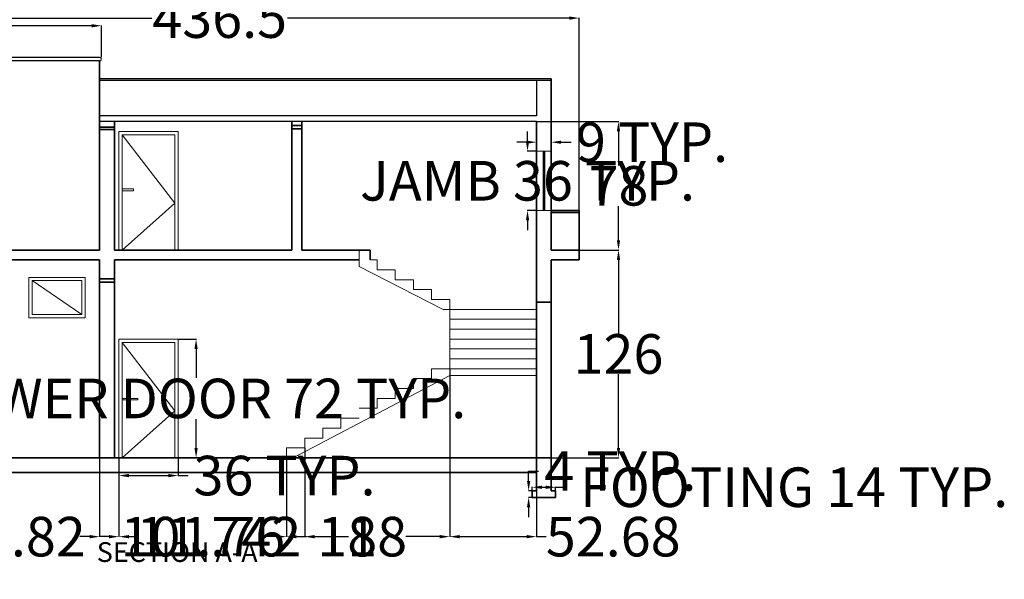
# Model space of a CAD drawing. Units: inches. Extents: x -15 to 1815, y 1023 to 2303.
# Tile 7 of 8: x 1217 to 1815, y 1433 to 1773. Entities that reach past the tile are written whole.
import ezdxf

# ---------------------------------------------------------------- set-up
doc = ezdxf.new("R2010")
doc.units = ezdxf.units.IN
doc.header["$MEASUREMENT"] = 0
for name, color, linetype, lineweight in [('A-ANNO-DIMS', 2, 'Continuous', 18), ('A-ANNO-TEXT', 7, 'Continuous', 25), ('A-DOOR', 3, 'Continuous', 18), ('A-FLOR', 7, 'Continuous', 35), ('A-FLOR-STRS', 3, 'Continuous', 18), ('A-GLAZ', 4, 'Continuous', 18), ('A-ROOF', 7, 'Continuous', 25), ('A-SECT', 7, 'Continuous', 35), ('S-FNDN', 7, 'Continuous', 35)]:
    doc.layers.add(name, color=color, linetype=linetype, lineweight=lineweight)
doc.styles.get("Standard").update_dxf_attribs({"font": 'arial.ttf'})
doc.dimstyles.get("Standard").update_dxf_attribs({"dimtxt": 24, "dimasz": 6, "dimexe": 0.18, "dimexo": 0.0625, "dimgap": 0.09, "dimtad": 0, "dimtih": 1, "dimtoh": 1, "dimdec": 0, "dimzin": 0, "dimdsep": 46, "dimlunit": 3, "dimtxsty": 'Standard', "dimcen": 0.09, "dimadec": 0, "dimazin": 0, "dimtfac": 1, "dimtdec": 0, "dimtofl": 0, "dimtmove": 0, "dimatfit": 3, "dimfxl": 1, "dimtolj": 1, "dimtzin": 0, "dimarcsym": 0})

# ---------------------------------------------------------------- blocks, each defined once
blk = doc.blocks.new('DOOR-36-SEC-LEVER')
for p, q in [((2, 70), (34, 28.45)), ((34, 28.45), (2, 0)), ((2, 2), (2, 0)), ((34, 2), (34, 0))]:
    blk.add_line(p, q)
for points in [[(0, 0), (36, 0), (36, 72), (0, 72)], [(2, 36), (11.36, 36), (11.36, 35.17), (2, 35.17)]]:
    blk.add_lwpolyline(points, close=True)
blk.add_lwpolyline([(34, 2), (34, 70), (2, 70), (2, 2)])
blk = doc.blocks.new('DOOR-36-SEC-RETURN-LEVER')
for p, q in [((2, 70), (34, 28.45)), ((8.91, 37.23), (2, 37.23)), ((8.91, 36), (2, 36)), ((8.91, 36), (8.91, 37.23)), ((34, 28.45), (2, 0)), ((2, 2), (2, 0)), ((34, 2), (34, 0))]:
    blk.add_line(p, q)
for points in [[(0, 0), (36, 0), (36, 72), (0, 72)], [(2, 36), (8.91, 36), (8.91, 36), (2, 36)]]:
    blk.add_lwpolyline(points, close=True)
blk.add_lwpolyline([(34, 2), (34, 70), (2, 70), (2, 2)])
blk = doc.blocks.new('WIN-AWNING-ELEV')
blk.add_line((32.26, 2), (2, 22.53))
for points in [[(0, 24.53), (34.26, 24.53), (34.26, 0), (0, 0)], [(2, 22.53), (32.26, 22.53), (32.26, 2), (2, 2)]]:
    blk.add_lwpolyline(points, close=True)
blk = doc.blocks.new('WIN-36-JAMB-SEC')
for p, q in [((4, 36.04), (4, 0)), ((4.5, 36.04), (4.5, 0)), ((5, 36.04), (5, 0))]:
    blk.add_line(p, q)
blk.add_lwpolyline([(9, 0), (0, 0), (0, 36.04), (9, 36.04)], close=True)
blk = doc.blocks.new('COPING-ROUND-END')
for p, q in [((1.07, 2.13), (126.89, 2.13)), ((1.07, 0), (126.89, 0))]:
    blk.add_line(p, q)
for centre, start, end in [((1.07, 1.07), 90, 270), ((126.89, 1.07), 270, 90)]:
    blk.add_arc(centre, 1.07, start, end)
blk = doc.blocks.new('FOOTING-STRIP-SECTION')
for p, q in [((0, 0), (0, 3.98)), ((0, 3.98), (2.61, 3.98)), ((14.22, 0), (0, 0)), ((14.22, 3.98), (11.61, 3.98)), ((14.22, 0), (14.22, 3.98))]:
    blk.add_line(p, q)
blk = doc.blocks.new('*D45')
at = {"layer": 'A-ANNO-DIMS', "color": 0, "lineweight": -2, "transparency": 16777216}
for p, q in [((1138.43, 1750.02), (1138.43, 1769.34)), ((1266.44, 1750.02), (1266.44, 1769.34)), ((1138.43, 1769.16), (1132.43, 1769.16)), ((1260.44, 1769.16), (1144.43, 1769.16))]:
    blk.add_line(p, q, dxfattribs=at)
at = {"layer": 'A-ANNO-DIMS', "color": 0, "transparency": 16777216}
for points in [[(1144.43, 1770.16), (1144.43, 1768.16), (1138.43, 1769.16)], [(1260.44, 1770.16), (1260.44, 1768.16), (1266.44, 1769.16)]]:
    blk.add_solid(points, dxfattribs=at)
at = {"layer": 'Defpoints', "color": 0, "transparency": 16777216}
for p in [(1138.43, 1769.16), (1138.43, 1749.96), (1266.44, 1749.96)]:
    blk.add_point(p, dxfattribs=at)
at = {"layer": 'A-ANNO-DIMS', "color": 0, "transparency": 16777216, "insert": (993.96, 1769.16), "char_height": 24, "attachment_point": 5}
blk.add_mtext('\\A1;COPING 128 TYP.', dxfattribs=at)
blk = doc.blocks.new('*D47')
at = {"layer": 'A-ANNO-DIMS', "color": 0, "lineweight": -2, "transparency": 16777216}
for p, q in [((1527.89, 1487.12), (1527.89, 1489.37)), ((1533.89, 1489.19), (1536.11, 1489.19)), ((1542.11, 1487.12), (1542.11, 1489.37)), ((1542.11, 1489.19), (1548.11, 1489.19))]:
    blk.add_line(p, q, dxfattribs=at)
at = {"layer": 'A-ANNO-DIMS', "color": 0, "transparency": 16777216}
for points in [[(1533.89, 1490.19), (1533.89, 1488.19), (1527.89, 1489.19)], [(1536.11, 1490.19), (1536.11, 1488.19), (1542.11, 1489.19)]]:
    blk.add_solid(points, dxfattribs=at)
at = {"layer": 'Defpoints', "color": 0, "transparency": 16777216}
for p in [(1542.11, 1489.19), (1527.89, 1487.06), (1542.11, 1487.06)]:
    blk.add_point(p, dxfattribs=at)
at = {"layer": 'A-ANNO-DIMS', "color": 0, "transparency": 16777216, "insert": (1686.95, 1489.19), "char_height": 24, "attachment_point": 5}
blk.add_mtext('\\A1;FOOTING 14 TYP.', dxfattribs=at)
blk = doc.blocks.new('*D48')
at = {"layer": 'A-ANNO-DIMS', "color": 0, "lineweight": -2, "transparency": 16777216}
for p, q in [((1525.76, 1493.06), (1525.76, 1499.06)), ((1525.76, 1499.06), (1531.76, 1499.06)), ((1527.83, 1487.06), (1525.58, 1487.06)), ((1527.83, 1483.08), (1525.58, 1483.08)), ((1525.76, 1477.08), (1525.76, 1471.08))]:
    blk.add_line(p, q, dxfattribs=at)
at = {"layer": 'A-ANNO-DIMS', "color": 0, "transparency": 16777216}
for points in [[(1524.76, 1493.06), (1526.76, 1493.06), (1525.76, 1487.06)], [(1524.76, 1477.08), (1526.76, 1477.08), (1525.76, 1483.08)]]:
    blk.add_solid(points, dxfattribs=at)
at = {"layer": 'Defpoints', "color": 0, "transparency": 16777216}
for p in [(1525.76, 1487.06), (1527.89, 1487.06), (1527.89, 1483.08)]:
    blk.add_point(p, dxfattribs=at)
at = {"layer": 'A-ANNO-DIMS', "color": 0, "transparency": 16777216, "insert": (1581.42, 1499.06), "char_height": 24, "attachment_point": 5}
blk.add_mtext('\\A1;4 TYP.', dxfattribs=at)
blk = doc.blocks.new('*D49')
at = {"layer": 'A-ANNO-DIMS', "color": 0, "lineweight": -2, "transparency": 16777216}
for p, q in [((1313.13, 1579.08), (1324.05, 1579.08)), ((1323.87, 1573.08), (1323.87, 1555.58)), ((1323.87, 1513.08), (1323.87, 1530.57)), ((1313.13, 1507.08), (1324.05, 1507.08))]:
    blk.add_line(p, q, dxfattribs=at)
at = {"layer": 'A-ANNO-DIMS', "color": 0, "transparency": 16777216}
for points in [[(1322.87, 1573.08), (1324.87, 1573.08), (1323.87, 1579.08)], [(1322.87, 1513.08), (1324.87, 1513.08), (1323.87, 1507.08)]]:
    blk.add_solid(points, dxfattribs=at)
at = {"layer": 'Defpoints', "color": 0, "transparency": 16777216}
for p in [(1313.07, 1579.08), (1323.87, 1579.08), (1313.07, 1507.08)]:
    blk.add_point(p, dxfattribs=at)
at = {"layer": 'A-ANNO-DIMS', "color": 0, "transparency": 16777216, "insert": (1323.87, 1543.08), "char_height": 24, "attachment_point": 5}
blk.add_mtext('\\A1;LOWER DOOR 72 TYP.', dxfattribs=at)
blk = doc.blocks.new('*D50')
at = {"layer": 'A-ANNO-DIMS', "color": 0, "lineweight": -2, "transparency": 16777216}
for p, q in [((1277.07, 1507.01), (1277.07, 1496.1)), ((1313.07, 1507.01), (1313.07, 1496.1)), ((1283.07, 1496.28), (1307.07, 1496.28)), ((1313.07, 1496.28), (1319.07, 1496.28))]:
    blk.add_line(p, q, dxfattribs=at)
at = {"layer": 'A-ANNO-DIMS', "color": 0, "transparency": 16777216}
for points in [[(1283.07, 1497.28), (1283.07, 1495.28), (1277.07, 1496.28)], [(1307.07, 1497.28), (1307.07, 1495.28), (1313.07, 1496.28)]]:
    blk.add_solid(points, dxfattribs=at)
at = {"layer": 'Defpoints', "color": 0, "transparency": 16777216}
for p in [(1277.07, 1507.08), (1313.07, 1507.08), (1313.07, 1496.28)]:
    blk.add_point(p, dxfattribs=at)
at = {"layer": 'A-ANNO-DIMS', "color": 0, "transparency": 16777216, "insert": (1377.56, 1496.28), "char_height": 24, "attachment_point": 5}
blk.add_mtext('\\A1;36 TYP.', dxfattribs=at)
blk = doc.blocks.new('*D55')
at = {"layer": 'A-ANNO-DIMS', "color": 0, "lineweight": -2, "transparency": 16777216}
for p, q in [((1525.09, 1699.11), (1525.09, 1705.11)), ((1530.44, 1693.11), (1524.91, 1693.11)), ((1530.44, 1657.08), (1524.91, 1657.08)), ((1525.09, 1651.08), (1525.09, 1645.08))]:
    blk.add_line(p, q, dxfattribs=at)
at = {"layer": 'A-ANNO-DIMS', "color": 0, "transparency": 16777216}
for points in [[(1524.09, 1699.11), (1526.09, 1699.11), (1525.09, 1693.11)], [(1524.09, 1651.08), (1526.09, 1651.08), (1525.09, 1657.08)]]:
    blk.add_solid(points, dxfattribs=at)
at = {"layer": 'Defpoints', "color": 0, "transparency": 16777216}
for p in [(1525.09, 1693.11), (1530.5, 1693.11), (1530.5, 1657.08)]:
    blk.add_point(p, dxfattribs=at)
at = {"layer": 'A-ANNO-DIMS', "color": 0, "transparency": 16777216, "insert": (1525.09, 1675.1), "char_height": 24, "attachment_point": 5}
blk.add_mtext('\\A1;JAMB 36 TYP.', dxfattribs=at)
blk = doc.blocks.new('*D56')
at = {"layer": 'A-ANNO-DIMS', "color": 0, "lineweight": -2, "transparency": 16777216}
for p, q in [((1524.5, 1698.52), (1518.5, 1698.52)), ((1530.5, 1693.18), (1530.5, 1698.7)), ((1539.5, 1693.18), (1539.5, 1698.7)), ((1545.5, 1698.52), (1551.5, 1698.52))]:
    blk.add_line(p, q, dxfattribs=at)
at = {"layer": 'A-ANNO-DIMS', "color": 0, "transparency": 16777216}
for points in [[(1524.5, 1699.52), (1524.5, 1697.52), (1530.5, 1698.52)], [(1545.5, 1699.52), (1545.5, 1697.52), (1539.5, 1698.52)]]:
    blk.add_solid(points, dxfattribs=at)
at = {"layer": 'Defpoints', "color": 0, "transparency": 16777216}
for p in [(1539.5, 1698.52), (1530.5, 1693.11), (1539.5, 1693.11)]:
    blk.add_point(p, dxfattribs=at)
at = {"layer": 'A-ANNO-DIMS', "color": 0, "transparency": 16777216, "insert": (1600.68, 1698.52), "char_height": 24, "attachment_point": 5}
blk.add_mtext('\\A1;9 TYP.', dxfattribs=at)
blk = doc.blocks.new('*D103')
at = {"layer": 'A-ANNO-DIMS', "color": 0, "lineweight": -2, "transparency": 16777216}
for p, q in [((1119.96, 1657.14), (1119.96, 1773.99)), ((1125.96, 1773.81), (1297.05, 1773.81)), ((1550.46, 1773.81), (1379.37, 1773.81)), ((1556.46, 1657.14), (1556.46, 1773.99))]:
    blk.add_line(p, q, dxfattribs=at)
at = {"layer": 'A-ANNO-DIMS', "color": 0, "transparency": 16777216}
for points in [[(1125.96, 1774.81), (1125.96, 1772.81), (1119.96, 1773.81)], [(1550.46, 1774.81), (1550.46, 1772.81), (1556.46, 1773.81)]]:
    blk.add_solid(points, dxfattribs=at)
at = {"layer": 'Defpoints', "color": 0, "transparency": 16777216}
for p in [(1556.46, 1773.81), (1119.96, 1657.08), (1556.46, 1657.08)]:
    blk.add_point(p, dxfattribs=at)
at = {"layer": 'A-ANNO-DIMS', "color": 0, "transparency": 16777216, "insert": (1338.21, 1773.81), "char_height": 24, "attachment_point": 5}
blk.add_mtext('\\A1;436.5', dxfattribs=at)
blk = doc.blocks.new('*D105')
at = {"layer": 'A-ANNO-DIMS', "color": 0, "lineweight": -2, "transparency": 16777216}
for p, q in [((1556.52, 1633.08), (1580.49, 1633.08)), ((1580.31, 1627.08), (1580.31, 1582.42)), ((1580.31, 1513.08), (1580.31, 1557.73)), ((1539.56, 1507.08), (1580.49, 1507.08))]:
    blk.add_line(p, q, dxfattribs=at)
at = {"layer": 'A-ANNO-DIMS', "color": 0, "transparency": 16777216}
for points in [[(1579.31, 1627.08), (1581.31, 1627.08), (1580.31, 1633.08)], [(1579.31, 1513.08), (1581.31, 1513.08), (1580.31, 1507.08)]]:
    blk.add_solid(points, dxfattribs=at)
at = {"layer": 'Defpoints', "color": 0, "transparency": 16777216}
for p in [(1556.46, 1633.08), (1580.31, 1633.08), (1539.5, 1507.08)]:
    blk.add_point(p, dxfattribs=at)
at = {"layer": 'A-ANNO-DIMS', "color": 0, "transparency": 16777216, "insert": (1580.31, 1570.08), "char_height": 24, "attachment_point": 5}
blk.add_mtext('\\A1;126', dxfattribs=at)
blk = doc.blocks.new('*D106')
at = {"layer": 'A-ANNO-DIMS', "color": 0, "lineweight": -2, "transparency": 16777216}
for p, q in [((1530.56, 1711.08), (1580.49, 1711.08)), ((1580.31, 1705.08), (1580.31, 1684.42)), ((1580.31, 1639.08), (1580.31, 1659.73)), ((1539.56, 1633.08), (1580.49, 1633.08))]:
    blk.add_line(p, q, dxfattribs=at)
at = {"layer": 'A-ANNO-DIMS', "color": 0, "transparency": 16777216}
for points in [[(1579.31, 1705.08), (1581.31, 1705.08), (1580.31, 1711.08)], [(1579.31, 1639.08), (1581.31, 1639.08), (1580.31, 1633.08)]]:
    blk.add_solid(points, dxfattribs=at)
at = {"layer": 'Defpoints', "color": 0, "transparency": 16777216}
for p in [(1530.5, 1711.08), (1580.31, 1711.08), (1539.5, 1633.08)]:
    blk.add_point(p, dxfattribs=at)
at = {"layer": 'A-ANNO-DIMS', "color": 0, "transparency": 16777216, "insert": (1580.31, 1672.08), "char_height": 24, "attachment_point": 5}
blk.add_mtext('\\A1;78', dxfattribs=at)
blk = doc.blocks.new('*D107')
at = {"layer": 'A-ANNO-DIMS', "color": 0, "lineweight": -2, "transparency": 16777216}
for p, q in [((1148.5, 1507.01), (1148.5, 1459.05)), ((1265.32, 1507.01), (1265.32, 1459.05)), ((1154.5, 1459.23), (1158.26, 1459.23)), ((1259.32, 1459.23), (1255.57, 1459.23))]:
    blk.add_line(p, q, dxfattribs=at)
at = {"layer": 'A-ANNO-DIMS', "color": 0, "transparency": 16777216}
for points in [[(1154.5, 1460.23), (1154.5, 1458.23), (1148.5, 1459.23)], [(1259.32, 1460.23), (1259.32, 1458.23), (1265.32, 1459.23)]]:
    blk.add_solid(points, dxfattribs=at)
at = {"layer": 'Defpoints', "color": 0, "transparency": 16777216}
for p in [(1148.5, 1507.08), (1265.32, 1507.08), (1265.32, 1459.23)]:
    blk.add_point(p, dxfattribs=at)
at = {"layer": 'A-ANNO-DIMS', "color": 0, "transparency": 16777216, "insert": (1206.91, 1459.23), "char_height": 24, "attachment_point": 5}
blk.add_mtext('\\A1;116.82', dxfattribs=at)
blk = doc.blocks.new('*D108')
at = {"layer": 'A-ANNO-DIMS', "color": 0, "lineweight": -2, "transparency": 16777216}
for p, q in [((1265.32, 1507.01), (1265.32, 1459.05)), ((1277.07, 1507.01), (1277.07, 1459.05)), ((1259.32, 1459.23), (1253.32, 1459.23)), ((1283.07, 1459.23), (1289.07, 1459.23))]:
    blk.add_line(p, q, dxfattribs=at)
at = {"layer": 'A-ANNO-DIMS', "color": 0, "transparency": 16777216}
for points in [[(1259.32, 1460.23), (1259.32, 1458.23), (1265.32, 1459.23)], [(1283.07, 1460.23), (1283.07, 1458.23), (1277.07, 1459.23)]]:
    blk.add_solid(points, dxfattribs=at)
at = {"layer": 'Defpoints', "color": 0, "transparency": 16777216}
for p in [(1265.32, 1507.08), (1277.07, 1507.08), (1277.07, 1459.23)]:
    blk.add_point(p, dxfattribs=at)
at = {"layer": 'A-ANNO-DIMS', "color": 0, "transparency": 16777216, "insert": (1337.72, 1459.23), "char_height": 24, "attachment_point": 5}
blk.add_mtext('\\A1;11.742', dxfattribs=at)
blk = doc.blocks.new('*D109')
at = {"layer": 'A-ANNO-DIMS', "color": 0, "lineweight": -2, "transparency": 16777216}
for p, q in [((1277.065913, 1507.014849), (1277.065913, 1459.047349)), ((1378.822077, 1507.014849), (1378.822077, 1459.047349)), ((1271.065913, 1459.227349), (1265.065913, 1459.227349)), ((1384.822077, 1459.227349), (1390.822077, 1459.227349))]:
    blk.add_line(p, q, dxfattribs=at)
at = {"layer": 'A-ANNO-DIMS', "color": 0, "transparency": 16777216}
for points in [[(1271.065913, 1460.227349), (1271.065913, 1458.227349), (1277.065913, 1459.227349)], [(1384.822077, 1460.227349), (1384.822077, 1458.227349), (1378.822077, 1459.227349)]]:
    blk.add_solid(points, dxfattribs=at)
at = {"layer": 'Defpoints', "color": 0, "transparency": 16777216}
for p in [(1277.065913, 1507.077349), (1378.822077, 1507.077349), (1378.822077, 1459.227349)]:
    blk.add_point(p, dxfattribs=at)
at = {"layer": 'A-ANNO-DIMS', "color": 0, "transparency": 16777216, "insert": (1327.943995, 1459.227349), "char_height": 24, "attachment_point": 5}
blk.add_mtext('\\A1;101.76', dxfattribs=at)
blk = doc.blocks.new('*D110')
at = {"layer": 'A-ANNO-DIMS', "color": 0, "lineweight": -2, "transparency": 16777216}
for p, q in [((1389.82, 1513.01), (1389.82, 1459.05)), ((1378.82, 1507.01), (1378.82, 1459.05)), ((1372.82, 1459.23), (1366.82, 1459.23)), ((1395.82, 1459.23), (1401.82, 1459.23))]:
    blk.add_line(p, q, dxfattribs=at)
at = {"layer": 'A-ANNO-DIMS', "color": 0, "transparency": 16777216}
for points in [[(1372.82, 1460.23), (1372.82, 1458.23), (1378.82, 1459.23)], [(1395.82, 1460.23), (1395.82, 1458.23), (1389.82, 1459.23)]]:
    blk.add_solid(points, dxfattribs=at)
at = {"layer": 'Defpoints', "color": 0, "transparency": 16777216}
for p in [(1389.82, 1513.08), (1378.82, 1507.08), (1389.82, 1459.23)]:
    blk.add_point(p, dxfattribs=at)
at = {"layer": 'A-ANNO-DIMS', "color": 0, "transparency": 16777216, "insert": (1415.66, 1459.23), "char_height": 24, "attachment_point": 5}
blk.add_mtext('\\A1;11', dxfattribs=at)
blk = doc.blocks.new('*D111')
at = {"layer": 'A-ANNO-DIMS', "color": 0, "lineweight": -2, "transparency": 16777216}
for p, q in [((1477.82, 1561.01), (1477.82, 1459.05)), ((1389.82, 1513.01), (1389.82, 1459.05)), ((1395.82, 1459.23), (1416.5, 1459.23)), ((1471.82, 1459.23), (1451.14, 1459.23))]:
    blk.add_line(p, q, dxfattribs=at)
at = {"layer": 'A-ANNO-DIMS', "color": 0, "transparency": 16777216}
for points in [[(1395.82, 1460.23), (1395.82, 1458.23), (1389.82, 1459.23)], [(1471.82, 1460.23), (1471.82, 1458.23), (1477.82, 1459.23)]]:
    blk.add_solid(points, dxfattribs=at)
at = {"layer": 'Defpoints', "color": 0, "transparency": 16777216}
for p in [(1477.82, 1561.08), (1389.82, 1513.08), (1477.82, 1459.23)]:
    blk.add_point(p, dxfattribs=at)
at = {"layer": 'A-ANNO-DIMS', "color": 0, "transparency": 16777216, "insert": (1433.82, 1459.23), "char_height": 24, "attachment_point": 5}
blk.add_mtext('\\A1;88', dxfattribs=at)
blk = doc.blocks.new('*D112')
at = {"layer": 'A-ANNO-DIMS', "color": 0, "lineweight": -2, "transparency": 16777216}
for p, q in [((1477.82, 1561.01), (1477.82, 1459.05)), ((1530.5, 1561.01), (1530.5, 1459.05)), ((1483.82, 1459.23), (1524.5, 1459.23)), ((1530.5, 1459.23), (1536.5, 1459.23))]:
    blk.add_line(p, q, dxfattribs=at)
at = {"layer": 'A-ANNO-DIMS', "color": 0, "transparency": 16777216}
for points in [[(1483.82, 1460.23), (1483.82, 1458.23), (1477.82, 1459.23)], [(1524.5, 1460.23), (1524.5, 1458.23), (1530.5, 1459.23)]]:
    blk.add_solid(points, dxfattribs=at)
at = {"layer": 'Defpoints', "color": 0, "transparency": 16777216}
for p in [(1477.82, 1561.08), (1530.5, 1561.08), (1530.5, 1459.23)]:
    blk.add_point(p, dxfattribs=at)
at = {"layer": 'A-ANNO-DIMS', "color": 0, "transparency": 16777216, "insert": (1577.11, 1459.23), "char_height": 24, "attachment_point": 5}
blk.add_mtext('\\A1;52.68', dxfattribs=at)

msp = doc.modelspace()

# ---------------------------------------------------------------- linework, layer by layer
at = {"layer": 'A-FLOR'}
for p, q in [((1556.4613, 1657.0773), (1539.4997, 1657.0773)), ((1556.4613, 1657.0773), (1539.4997, 1657.0773)), ((1556.4613, 1655.9681), (1539.4997, 1655.9681)), ((1556.4613, 1657.0773), (1556.4613, 1627.0773)), ((1265.3241, 1633.0773), (1139.4997, 1633.0773)), ((1382.0448, 1633.0773), (1274.3241, 1633.0773)), ((1428.66, 1633.0773), (1388.0448, 1633.0773)), ((1429.568, 1633.0773), (1388.9528, 1633.0773)), ((1429.568, 1633.0773), (1429.568, 1627.0773)), ((1556.4613, 1633.0773), (1539.4997, 1633.0773)), ((1265.3241, 1627.0773), (1139.4997, 1627.0773)), ((1422.8221, 1627.0773), (1274.3241, 1627.0773)), ((1556.4613, 1627.0773), (1539.4997, 1627.0773)), ((1265.3241, 1507.0773), (1139.4997, 1507.0773)), ((1539.4997, 1507.0773), (1265.3241, 1507.0773)), ((1265.3241, 1498.0773), (1148.4997, 1498.0773)), ((1530.4997, 1498.0773), (1265.3241, 1498.0773))]:
    msp.add_line(p, q, dxfattribs=at)
at = {"layer": 'A-FLOR-STRS'}
for p, q in [((1422.8221, 1623.0773), (1422.8221, 1633.0773)), ((1433.8221, 1627.0773), (1429.568, 1627.0773)), ((1433.8221, 1621.0773), (1433.8221, 1627.0773)), ((1473.8221, 1597.0773), (1422.8221, 1623.0773)), ((1444.8221, 1621.0773), (1433.8221, 1621.0773)), ((1444.8221, 1615.0773), (1444.8221, 1621.0773)), ((1455.8221, 1615.0773), (1444.8221, 1615.0773)), ((1455.8221, 1609.0773), (1455.8221, 1615.0773)), ((1466.8221, 1609.0773), (1455.8221, 1609.0773)), ((1466.8221, 1603.0773), (1466.8221, 1609.0773)), ((1477.8221, 1603.0773), (1466.8221, 1603.0773)), ((1477.8221, 1597.0773), (1477.8221, 1603.0773)), ((1477.8221, 1597.0773), (1473.8221, 1597.0773)), ((1477.8221, 1597.0773), (1530.4997, 1597.0773)), ((1477.8221, 1561.0773), (1477.8221, 1597.0773)), ((1477.8221, 1591.0773), (1530.4997, 1591.0773)), ((1477.8221, 1585.0773), (1530.4997, 1585.0773)), ((1477.8221, 1579.0773), (1530.4997, 1579.0773)), ((1477.8221, 1573.0773), (1530.4997, 1573.0773)), ((1477.8221, 1567.0773), (1530.4997, 1567.0773)), ((1466.8221, 1555.0773), (1466.8221, 1561.0773)), ((1466.8221, 1561.0773), (1477.8221, 1561.0773)), ((1477.8221, 1561.0773), (1530.4997, 1561.0773)), ((1477.8221, 1557.0773), (1382.8221, 1507.0773)), ((1455.8221, 1549.0773), (1455.8221, 1555.0773)), ((1455.8221, 1555.0773), (1466.8221, 1555.0773)), ((1477.8221, 1557.0773), (1530.4997, 1557.0773)), ((1444.8221, 1543.0773), (1444.8221, 1549.0773)), ((1444.8221, 1549.0773), (1455.8221, 1549.0773)), ((1433.8221, 1537.0773), (1433.8221, 1543.0773)), ((1433.8221, 1543.0773), (1444.8221, 1543.0773)), ((1422.8221, 1537.0773), (1433.8221, 1537.0773)), ((1411.8221, 1525.0773), (1411.8221, 1531.0773)), ((1411.8221, 1531.0773), (1422.8221, 1531.0773)), ((1400.8221, 1519.0773), (1400.8221, 1525.0773)), ((1400.8221, 1525.0773), (1411.8221, 1525.0773)), ((1389.8221, 1513.0773), (1389.8221, 1519.0773)), ((1389.8221, 1519.0773), (1400.8221, 1519.0773)), ((1378.8221, 1507.0773), (1378.8221, 1513.0773)), ((1378.8221, 1513.0773), (1389.8221, 1513.0773))]:
    msp.add_line(p, q, dxfattribs=at)
at = {"layer": 'A-ROOF'}
for p, q in [((1539.4997, 1736.9695), (1265.3241, 1736.9695)), ((1539.4997, 1735.8674), (1265.3241, 1735.8674)), ((1530.4997, 1735.8674), (1530.4997, 1714.6079)), ((1530.4997, 1714.6079), (1265.3241, 1714.6079)), ((1530.4997, 1711.0773), (1265.3241, 1711.0773))]:
    msp.add_line(p, q, dxfattribs=at)
at = {"layer": 'A-SECT'}
for p, q in [((1265.3241, 1711.0773), (1265.3241, 1747.8268)), ((1539.4997, 1736.9695), (1539.4997, 1633.0773)), ((1265.3241, 1711.0773), (1265.3241, 1633.0773)), ((1274.3241, 1711.0773), (1274.3241, 1633.0773)), ((1382.0448, 1711.0773), (1382.0448, 1633.0773)), ((1388.0448, 1711.0773), (1388.0448, 1633.0773)), ((1530.4997, 1711.0773), (1530.4997, 1607.8282)), ((1265.3241, 1627.0773), (1265.3241, 1507.0773)), ((1274.3241, 1627.0773), (1274.3241, 1507.0773)), ((1539.4997, 1627.0773), (1539.4997, 1607.8282)), ((1530.4997, 1607.8282), (1530.4997, 1507.0773)), ((1539.4997, 1607.8282), (1539.4997, 1507.0773)), ((1530.4997, 1601.4023), (1539.4997, 1601.4023))]:
    msp.add_line(p, q, dxfattribs=at)
for points in [[(1265.3241, 1707.6644), (1274.3241, 1707.6644), (1274.3241, 1706.2986), (1265.3241, 1706.2986)], [(1382.0448, 1708.6419), (1388.0448, 1708.6419), (1388.0448, 1706.702), (1382.0448, 1706.702)], [(1265.3241, 1615.7133), (1274.3241, 1615.7133), (1274.3241, 1613.5418), (1265.3241, 1613.5418)]]:
    msp.add_lwpolyline(points, close=True, dxfattribs=at)
at = {"layer": 'S-FNDN'}
for p, q in [((1530.4997, 1582.655), (1530.4997, 1487.0609)), ((1530.4997, 1582.655), (1530.4997, 1487.0609)), ((1539.4997, 1582.655), (1539.4997, 1487.0609)), ((1539.4997, 1483.0773), (1527.8895, 1483.0773))]:
    msp.add_line(p, q, dxfattribs=at)

# ---------------------------------------------------------------- block references
at = {"layer": 'A-DOOR'}
for name, p in [('DOOR-36-SEC-RETURN-LEVER', (1277.0659, 1633.0773)), ('DOOR-36-SEC-LEVER', (1277.0659, 1507.0773))]:
    msp.add_blockref(name, p, dxfattribs=at)
at = {"layer": 'A-GLAZ'}
for name, p in [('WIN-36-JAMB-SEC', (1530.4997, 1657.0773)), ('WIN-AWNING-ELEV', (1222.3022, 1592.0097))]:
    msp.add_blockref(name, p, dxfattribs=at)
at = {"layer": 'A-ROOF', "rotation": 180}
msp.add_blockref('COPING-ROUND-END', (1266.39, 1749.9585), dxfattribs=at)
at = {"layer": 'S-FNDN'}
msp.add_blockref('FOOTING-STRIP-SECTION', (1527.8895, 1483.0773), dxfattribs=at)

# ---------------------------------------------------------------- texts
at = {"layer": 'A-ANNO-TEXT'}
msp.add_text('SECTION A-A', height=12, dxfattribs=at).set_placement((1263.5542, 1443.8867))

# ---------------------------------------------------------------- dimensions: what is measured, and where the dimension line sits
at = {"layer": 'A-ANNO-DIMS'}
for base, p1, p2, angle, text, picture, middle in [((1138.4338, 1769.1591), (1266.4376, 1749.9585), (1138.4338, 1749.9585), 180, 'COPING <> TYP.', '*D45', (993.9591, 1769.1591)), ((1525.0943, 1693.1133), (1530.4997, 1657.0773), (1530.4997, 1693.1133), 90, 'JAMB <> TYP.', '*D55', (1525.0943, 1675.0953)), ((1323.8659, 1579.0773), (1313.0659, 1507.0773), (1313.0659, 1579.0773), 90, 'LOWER DOOR <> TYP.', '*D49', (1323.8659, 1543.0773)), ((1525.7565, 1487.0609), (1527.8895, 1483.0773), (1527.8895, 1487.0609), 90, '<> TYP.', '*D48', (1581.4181, 1499.0609))]:
    dim = msp.add_linear_dim(base=base, p1=p1, p2=p2, angle=angle, text=text, dimstyle='Standard', override={"dimdec": 0, "dimlfac": 1, "dimrnd": 0, "dimzin": 0, "dimdsep": 46, "dimlunit": 2}, dxfattribs=at)
    dim.commit()
    dim.dimension.update_dxf_attribs({"geometry": picture, "text_midpoint": middle})
for base, p1, p2, override, picture, middle in [((1556.4613, 1773.8085), (1119.956, 1657.0773), (1556.4613, 1657.0773), {"dimdec": 1, "dimlfac": 1, "dimrnd": 0, "dimzin": 0, "dimdsep": 46, "dimlunit": 2}, '*D103', (1338.2086, 1773.8085)), ((1477.8221, 1459.2273), (1389.8221, 1513.0773), (1477.8221, 1561.0773), {"dimdec": 0, "dimlfac": 1, "dimrnd": 0, "dimzin": 0, "dimdsep": 46, "dimlunit": 2}, '*D111', (1433.8221, 1459.2273)), ((1530.4997, 1459.2273), (1477.8221, 1561.0773), (1530.4997, 1561.0773), {"dimdec": 2, "dimlfac": 1, "dimrnd": 0, "dimzin": 0, "dimdsep": 46, "dimlunit": 2}, '*D112', (1577.1081, 1459.2273)), ((1389.8221, 1459.2273), (1378.8221, 1507.0773), (1389.8221, 1513.0773), {"dimdec": 0, "dimlfac": 1, "dimrnd": 0, "dimzin": 0, "dimdsep": 46, "dimlunit": 2}, '*D110', (1415.6556, 1459.2273)), ((1265.3241, 1459.2273), (1148.4997, 1507.0773), (1265.3241, 1507.0773), {"dimdec": 2, "dimlfac": 1, "dimrnd": 0, "dimzin": 0, "dimdsep": 46, "dimlunit": 2}, '*D107', (1206.9119, 1459.2273)), ((1277.0659, 1459.2273), (1265.3241, 1507.0773), (1277.0659, 1507.0773), {"dimdec": 3, "dimlfac": 1, "dimrnd": 0, "dimzin": 0, "dimdsep": 46, "dimlunit": 2}, '*D108', (1337.7207, 1459.2273)), ((1378.8221, 1459.2273), (1277.0659, 1507.0773), (1378.8221, 1507.0773), {"dimdec": 2, "dimlfac": 1, "dimrnd": 0, "dimzin": 0, "dimdsep": 46, "dimlunit": 2}, '*D109', (1327.944, 1459.2273))]:
    dim = msp.add_linear_dim(base=base, p1=p1, p2=p2, dimstyle='Standard', override=override, dxfattribs=at)
    dim.commit()
    dim.dimension.update_dxf_attribs({"geometry": picture, "text_midpoint": middle})
for base, p1, p2, text, picture, middle in [((1539.4997, 1698.5187), (1530.4997, 1693.1133), (1539.4997, 1693.1133), '<> TYP.', '*D56', (1600.6783, 1698.5187)), ((1542.1098, 1489.1939), (1527.8895, 1487.0609), (1542.1098, 1487.0609), 'FOOTING <> TYP.', '*D47', (1686.9528, 1489.1939)), ((1313.0659, 1496.2773), (1277.0659, 1507.0773), (1313.0659, 1507.0773), '<> TYP.', '*D50', (1377.5597, 1496.2773))]:
    dim = msp.add_linear_dim(base=base, p1=p1, p2=p2, text=text, dimstyle='Standard', override={"dimdec": 0, "dimlfac": 1, "dimrnd": 0, "dimzin": 0, "dimdsep": 46, "dimlunit": 2}, dxfattribs=at)
    dim.commit()
    dim.dimension.update_dxf_attribs({"geometry": picture, "text_midpoint": middle})
for base, p1, p2, picture, middle in [((1580.3113, 1711.0773), (1539.4997, 1633.0773), (1530.4997, 1711.0773), '*D106', (1580.3113, 1672.0773)), ((1580.3113, 1633.0773), (1539.4997, 1507.0773), (1556.4613, 1633.0773), '*D105', (1580.3113, 1570.0773))]:
    dim = msp.add_linear_dim(base=base, p1=p1, p2=p2, angle=90, dimstyle='Standard', override={"dimdec": 0, "dimlfac": 1, "dimrnd": 0, "dimzin": 0, "dimdsep": 46, "dimlunit": 2}, dxfattribs=at)
    dim.commit()
    dim.dimension.update_dxf_attribs({"geometry": picture, "text_midpoint": middle})

doc.saveas('drawing.dxf')
